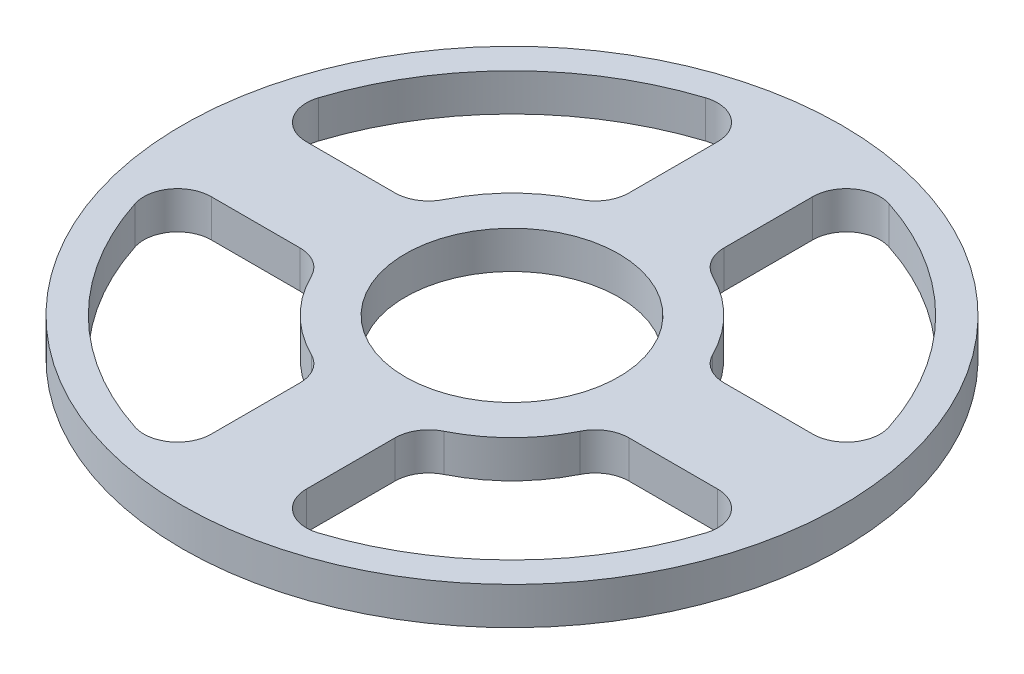
from build123d import *

# Parameters (mm, degrees)
WEB_DISC_PROFILE_90_R                  = 44
WEB_DISC_90X5_DEPTH                    = 5
BORE_AND_SPOKE_WINDOWS_PROFILE_R       = 14.25
CENTRE_BORE_AND_4X_SPOKE_WINDOWS_DEPTH = 44


with BuildPart() as part:
    # Web Disc Profile Ø90 → Web Disc Ø90x5 (new body)
    with BuildSketch(Plane(origin=(0, 0, 0), x_dir=(1, 0, 0), z_dir=(0, 1, 0))):
        with Locations(Location((0, 0, 0), (0, 0, 270))):
            Circle(WEB_DISC_PROFILE_90_R)
    extrude(amount=WEB_DISC_90X5_DEPTH)

    # Bore and Spoke Windows Profile → Centre Bore and 4x Spoke Windows (cut)
    with BuildSketch(Plane(origin=(0, 5, 0), x_dir=(1, 0, 0), z_dir=(0, 1, 0))):
        with BuildLine():
            Line((-21.966508598, 6.35), (-33.801294354, 6.35))
            ThreePointArc((-33.801294354, 6.35), (-37.437163198, 8.198498964), (-38.085965469, 12.225352113))
            ThreePointArc((-38.085965469, 12.225352113), (-28.284271247, 28.284271247), (-12.225352113, 38.085965469))
            ThreePointArc((-12.225352113, 38.085965469), (-8.198498964, 37.437163198), (-6.35, 33.801294354))
            Line((-6.35, 33.801294354), (-6.35, 21.966508598))
            ThreePointArc((-6.35, 21.966508598), (-7.027837187, 19.591414615), (-8.857142857, 17.931843754))
            ThreePointArc((-8.857142857, 17.931843754), (-14.142135624, 14.142135624), (-17.931843754, 8.857142857))
            ThreePointArc((-17.931843754, 8.857142857), (-19.591414615, 7.027837187), (-21.966508598, 6.35))
        make_face()
        with BuildLine():
            Line((21.966508598, 6.35), (33.801294354, 6.35))
            ThreePointArc((33.801294354, 6.35), (37.437163198, 8.198498964), (38.085965469, 12.225352113))
            ThreePointArc((38.085965469, 12.225352113), (28.284271247, 28.284271247), (12.225352113, 38.085965469))
            ThreePointArc((12.225352113, 38.085965469), (8.198498964, 37.437163198), (6.35, 33.801294354))
            Line((6.35, 33.801294354), (6.35, 21.966508598))
            ThreePointArc((6.35, 21.966508598), (7.027837187, 19.591414615), (8.857142857, 17.931843754))
            ThreePointArc((8.857142857, 17.931843754), (14.142135624, 14.142135624), (17.931843754, 8.857142857))
            ThreePointArc((17.931843754, 8.857142857), (19.591414615, 7.027837187), (21.966508598, 6.35))
        make_face()
        with BuildLine():
            Line((21.966508598, -6.35), (33.801294354, -6.35))
            ThreePointArc((33.801294354, -6.35), (37.437163198, -8.198498964), (38.085965469, -12.225352113))
            ThreePointArc((38.085965469, -12.225352113), (28.284271247, -28.284271247), (12.225352113, -38.085965469))
            ThreePointArc((12.225352113, -38.085965469), (8.198498964, -37.437163198), (6.35, -33.801294354))
            Line((6.35, -33.801294354), (6.35, -21.966508598))
            ThreePointArc((6.35, -21.966508598), (7.027837187, -19.591414615), (8.857142857, -17.931843754))
            ThreePointArc((8.857142857, -17.931843754), (14.142135624, -14.142135624), (17.931843754, -8.857142857))
            ThreePointArc((17.931843754, -8.857142857), (19.591414615, -7.027837187), (21.966508598, -6.35))
        make_face()
        with BuildLine():
            Line((-6.35, -21.966508598), (-6.35, -33.801294354))
            ThreePointArc((-6.35, -33.801294354), (-8.198498964, -37.437163198), (-12.225352113, -38.085965469))
            ThreePointArc((-12.225352113, -38.085965469), (-28.284271247, -28.284271247), (-38.085965469, -12.225352113))
            ThreePointArc((-38.085965469, -12.225352113), (-37.437163198, -8.198498964), (-33.801294354, -6.35))
            Line((-33.801294354, -6.35), (-21.966508598, -6.35))
            ThreePointArc((-21.966508598, -6.35), (-19.591414615, -7.027837187), (-17.931843754, -8.857142857))
            ThreePointArc((-17.931843754, -8.857142857), (-14.142135624, -14.142135624), (-8.857142857, -17.931843754))
            ThreePointArc((-8.857142857, -17.931843754), (-7.027837187, -19.591414615), (-6.35, -21.966508598))
        make_face()
        with Locations(Location((0, 0, 0), (0, 0, 270))):
            Circle(BORE_AND_SPOKE_WINDOWS_PROFILE_R)
    extrude(amount=-CENTRE_BORE_AND_4X_SPOKE_WINDOWS_DEPTH, mode=Mode.SUBTRACT)


solid = part.part
